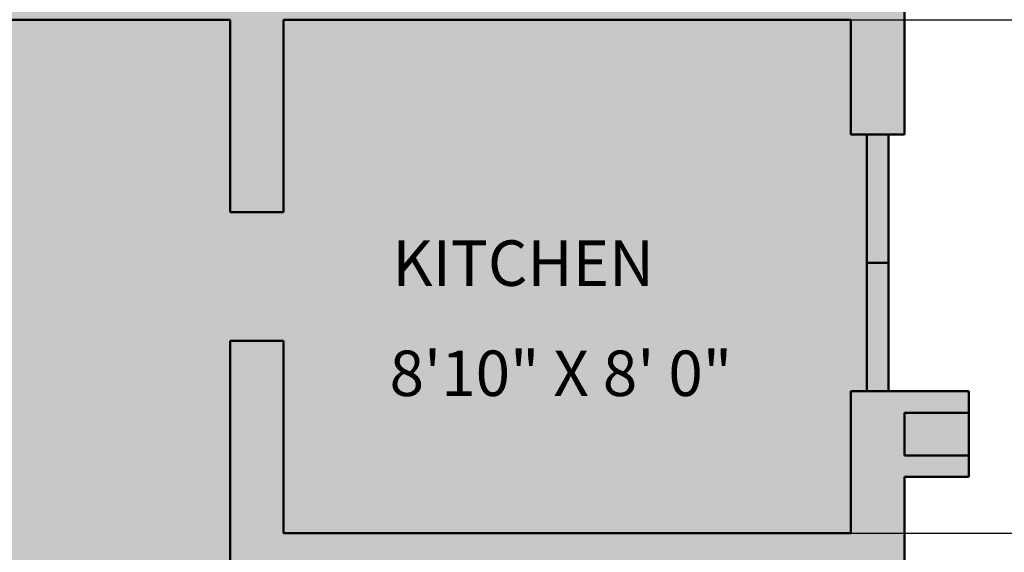
# Model space of a CAD drawing. Units: inches. Extents: x 925 to 2834, y 111 to 1355.
# Tile 19 of 25: x 1553 to 1737, y 972 to 1072. Entities that reach past the tile are written whole.
import ezdxf

# ---------------------------------------------------------------- set-up
doc = ezdxf.new("R2010")
doc.units = ezdxf.units.IN
doc.header["$MEASUREMENT"] = 0
for name, color, linetype, lineweight in [('A-ANNO-DIMS', 2, 'Continuous', 18), ('A-AREA-IDEN', 7, 'Continuous', 18), ('A-FLOR-PATT', 252, 'Continuous', 13), ('A-WALL', 7, 'Continuous', 50), ('A-WALL-PATT', 8, 'Continuous', 13)]:
    doc.layers.add(name, color=color, linetype=linetype, lineweight=lineweight)
doc.styles.get("Standard").update_dxf_attribs({"font": 'arial.ttf'})
doc.dimstyles.get("Standard").update_dxf_attribs({"dimtxt": 6, "dimasz": 3, "dimexe": 0.18, "dimexo": 0.0625, "dimgap": 0.09, "dimtad": 0, "dimtih": 1, "dimtoh": 1, "dimdec": 1, "dimzin": 0, "dimdsep": 46, "dimlunit": 3, "dimtxsty": 'Standard', "dimblk": 'ARCHTICK', "dimcen": 0.09, "dimadec": 0, "dimazin": 0, "dimtfac": 1, "dimtdec": 1, "dimtofl": 0, "dimtmove": 0, "dimatfit": 3, "dimfxl": 1, "dimtolj": 1, "dimtzin": 0, "dimarcsym": 0})

# ---------------------------------------------------------------- blocks, each defined once
blk = doc.blocks.new('_ArchTick')
at = {"color": 0, "linetype": 'ByBlock', "const_width": 0.15}
blk.add_lwpolyline([(-0.5, -0.5), (0.5, 0.5)], dxfattribs=at)
blk = doc.blocks.new('*D48')
at = {"layer": 'A-ANNO-DIMS', "color": 0, "lineweight": -2, "transparency": 16777216}
for p, q in [((1708.78, 975.59), (1988.62, 975.59)), ((1988.44, 975.59), (1988.44, 942.69)), ((1988.44, 903.59), (1988.44, 936.49)), ((1708.78, 903.59), (1988.62, 903.59))]:
    blk.add_line(p, q, dxfattribs=at)
at = {"layer": 'Defpoints', "color": 0, "transparency": 16777216}
for p in [(1708.71, 975.59), (1988.44, 975.59), (1708.71, 903.59)]:
    blk.add_point(p, dxfattribs=at)
at = {"layer": 'A-ANNO-DIMS', "color": 0, "lineweight": -2, "transparency": 16777216, "xscale": 3, "yscale": 3, "zscale": 3}
for p, rotation in [((1988.44, 975.59), 90), ((1988.44, 903.59), 270)]:
    blk.add_blockref('_ArchTick', p, dxfattribs=dict(at, rotation=rotation))
at = {"layer": 'A-ANNO-DIMS', "color": 0, "transparency": 16777216, "insert": (1988.44, 939.59), "char_height": 6, "attachment_point": 5}
blk.add_mtext('\\A1;72', dxfattribs=at)
blk = doc.blocks.new('*D49')
at = {"layer": 'A-ANNO-DIMS', "color": 0, "lineweight": -2, "transparency": 16777216}
for p, q in [((1708.78, 1071.59), (1988.62, 1071.59)), ((1988.44, 1071.59), (1988.44, 1026.74)), ((1988.44, 975.59), (1988.44, 1020.44)), ((1708.78, 975.59), (1988.62, 975.59))]:
    blk.add_line(p, q, dxfattribs=at)
at = {"layer": 'Defpoints', "color": 0, "transparency": 16777216}
for p in [(1708.71, 1071.59), (1988.44, 1071.59), (1708.71, 975.59)]:
    blk.add_point(p, dxfattribs=at)
at = {"layer": 'A-ANNO-DIMS', "color": 0, "lineweight": -2, "transparency": 16777216, "xscale": 3, "yscale": 3, "zscale": 3}
for p, rotation in [((1988.44, 1071.59), 90), ((1988.44, 975.59), 270)]:
    blk.add_blockref('_ArchTick', p, dxfattribs=dict(at, rotation=rotation))
at = {"layer": 'A-ANNO-DIMS', "color": 0, "transparency": 16777216, "insert": (1988.44, 1023.59), "char_height": 6, "attachment_point": 5}
blk.add_mtext('\\A1;96', dxfattribs=at)
blk = doc.blocks.new('*D50')
at = {"layer": 'A-ANNO-DIMS', "color": 0, "lineweight": -2, "transparency": 16777216}
for p, q in [((1718.78, 1081.59), (1988.62, 1081.59)), ((1988.44, 1081.59), (1988.44, 1079.74)), ((1988.44, 1071.59), (1988.44, 1073.44)), ((1708.78, 1071.59), (1988.62, 1071.59))]:
    blk.add_line(p, q, dxfattribs=at)
at = {"layer": 'Defpoints', "color": 0, "transparency": 16777216}
for p in [(1718.71, 1081.59), (1988.44, 1081.59), (1708.71, 1071.59)]:
    blk.add_point(p, dxfattribs=at)
at = {"layer": 'A-ANNO-DIMS', "color": 0, "lineweight": -2, "transparency": 16777216, "xscale": 3, "yscale": 3, "zscale": 3}
for p, rotation in [((1988.44, 1081.59), 90), ((1988.44, 1071.59), 270)]:
    blk.add_blockref('_ArchTick', p, dxfattribs=dict(at, rotation=rotation))
at = {"layer": 'A-ANNO-DIMS', "color": 0, "transparency": 16777216, "insert": (1988.44, 1076.59), "char_height": 6, "attachment_point": 5}
blk.add_mtext('\\A1;10', dxfattribs=at)

msp = doc.modelspace()

# ---------------------------------------------------------------- hatches: boundary and pattern name
at = {"layer": 'A-FLOR-PATT', "transparency": 33554605}
h = msp.add_hatch(color=256, dxfattribs=at)
h.dxf.hatch_style = 1
h.paths.add_polyline_path([(1931.688, 1294.5638), (991.7375, 1294.5638), (991.7375, 172.1134), (1931.688, 172.1134)])
h.paths.add_polyline_path([(1910.7128, 1273.5886), (1910.7128, 193.0886), (1012.7128, 193.0886), (1012.7128, 1273.5886)], flags=16)
h.paths.add_polyline_path([(1850.7128, 1213.5886), (1850.7128, 253.0886), (1072.7128, 253.0886), (1072.7128, 1213.5886)], flags=0)
h.paths.add_polyline_path([(1838.7128, 1201.5886), (1838.7128, 265.0886), (1084.7128, 265.0886), (1084.7128, 530.5886), (1084.7128, 1201.5886)], flags=0)
h.paths.add_polyline_path([(1547.6758, 1155.7396), (1547.6758, 1119.115), (1513.0687, 1119.115), (1513.0687, 1155.7396)], flags=0)
h.paths.add_polyline_path([(1600.1067, 1154.9439), (1634.7139, 1154.9439), (1634.7139, 1119.115), (1600.1067, 1119.115)], flags=0)
h.paths.add_polyline_path([(1505.2502, 1144.5358), (1505.2502, 1119.115), (1470.643, 1119.115), (1470.643, 1144.5358)], flags=0)
h.paths.add_polyline_path([(1559.1357, 1141.0962), (1593.7428, 1141.0962), (1593.7428, 1119.115), (1559.1357, 1119.115)], flags=0)
h.paths.add_polyline_path([(1462.8966, 1154.9439), (1462.8966, 1119.115), (1428.2895, 1119.115), (1428.2895, 1154.9439)], flags=0)
h.paths.add_polyline_path([(1642.4603, 1144.5358), (1677.0675, 1144.5358), (1677.0675, 1119.115), (1642.4603, 1119.115)], flags=0)
h.paths.add_polyline_path([(1422.3508, 1141.0962), (1422.3508, 1119.115), (1387.7436, 1119.115), (1387.7436, 1141.0962)], flags=0)
h.paths.add_polyline_path([(1684.8859, 1155.7396), (1719.4931, 1155.7396), (1719.4931, 1119.115), (1684.8859, 1119.115)], flags=0)
h.paths.add_polyline_path([(1718.7128, 1081.5886), (1718.7128, 1050.1249), (1715.7128, 1050.1249), (1715.7128, 1026.1249), (1715.7128, 1002.1249), (1718.7128, 1002.1249), (1730.7128, 1002.1249), (1730.7128, 998.1249), (1730.7128, 990.1249), (1730.7128, 986.1249), (1718.7128, 986.1249), (1718.7128, 893.5886), (1715.3735, 893.5886), (1715.3735, 891.5886), (1713.3735, 891.5886, 0.41421356), (1677.3735, 855.5886), (1713.3735, 855.5886), (1713.3735, 853.5886), (1715.3735, 853.5886), (1715.3735, 851.5886), (1718.7128, 851.5886), (1718.7128, 821.5865), (1734.4655, 821.5865), (1734.3735, 819.5886, -0.41421356), (1712.4415, 793.5886), (1712.4415, 791.5886), (1718.7128, 791.5886), (1718.7128, 717.5886), (1718.7128, 669.5886), (1732.7128, 669.5886), (1732.7128, 665.5886), (1732.7128, 641.5886), (1732.7128, 634.5886), (1732.7128, 610.5886), (1732.7128, 603.5886), (1718.7128, 603.5886), (1718.7128, 385.0886), (1434.2128, 385.0886), (1434.2128, 530.5886), (1410.2128, 530.5886), (1408.2128, 530.5886), (1408.2128, 532.5886, 0.41421356), (1372.2128, 568.5886), (1372.2128, 532.5886), (1370.2128, 532.5886), (1370.2128, 530.5886), (1368.2128, 530.5886), (1282.2128, 530.5886), (1210.2128, 530.5886), (1200.2128, 530.5886), (1200.2128, 542.1915), (1183.2307, 542.1915), (1183.2307, 546.1915), (1200.2128, 546.1915), (1200.2128, 572.1915), (1183.2307, 572.1915), (1183.2307, 576.1915), (1200.2128, 576.1915), (1200.2128, 727.5886), (1210.2128, 727.5886), (1234.2128, 727.5886), (1259.7128, 727.5886), (1259.7128, 775.5886), (1259.7128, 799.5886), (1259.7128, 847.5886), (1259.7128, 993.5872), (1259.7128, 1065.5872), (1259.7128, 1071.5886), (1219.6318, 1071.5886), (1219.6318, 1081.5886), (1084.7128, 1081.5886), (1084.7128, 1119.115), (1256.8974, 1119.115), (1256.8974, 1154.9439), (1291.5046, 1154.9439), (1291.5046, 1119.115), (1256.8974, 1119.115), (1256.6723, 1081.5886), (1293.7128, 1081.5886), (1341.7128, 1081.5886), (1341.7128, 1093.5886), (1347.7128, 1093.5886), (1371.7128, 1093.5886), (1377.7128, 1093.5886), (1377.7128, 1081.5886), (1668.7128, 1081.5886), (1668.7128, 1117.5886), (1675.7128, 1117.5886), (1711.7128, 1117.5886), (1718.7128, 1117.5886)], flags=0)
h.paths.add_polyline_path([(1376.2838, 1155.7396), (1376.2838, 1119.115), (1341.6766, 1119.115), (1341.6766, 1155.7396)], flags=0)
h.paths.add_polyline_path([(1341.7128, 1076.0886), (1293.7128, 1076.0886), (1293.7128, 1071.5886), (1269.7128, 1071.5886), (1269.7128, 1065.5872), (1266.7128, 1065.5872), (1266.7128, 1029.5872), (1265.7128, 1029.5872), (1265.7128, 993.5872), (1269.7128, 993.5872), (1269.7128, 903.5886), (1269.7128, 893.5886), (1269.7128, 847.5886), (1265.2128, 847.5886), (1265.2128, 799.5886), (1269.7128, 799.5886), (1269.7128, 775.5886), (1265.2128, 775.5886), (1265.2128, 727.5886), (1269.7128, 727.5886), (1444.2128, 727.5886), (1444.2128, 717.5886), (1234.2128, 717.5886), (1234.2128, 722.0886), (1210.2128, 722.0886), (1210.2128, 717.5886), (1210.2128, 540.5886), (1210.2128, 536.0886), (1282.2128, 536.0886), (1282.2128, 535.0886), (1210.2128, 535.0886), (1210.2128, 540.5886), (1210.2128, 717.5886), (1210.2128, 723.0886), (1234.2128, 723.0886), (1234.2128, 717.5886), (1444.2128, 717.5886), (1444.2128, 727.5886), (1269.7128, 727.5886), (1264.2128, 727.5886), (1264.2128, 775.5886), (1269.7128, 775.5886), (1269.7128, 799.5886), (1264.2128, 799.5886), (1264.2128, 847.5886), (1269.7128, 847.5886), (1269.7128, 893.5886), (1269.7128, 903.5886), (1269.7128, 993.5872), (1264.7128, 993.5872), (1264.7128, 1029.5872), (1265.7128, 1029.5872), (1265.7128, 1065.5872), (1269.7128, 1065.5872), (1269.7128, 1071.5886), (1293.7128, 1071.5886), (1293.7128, 1077.0886), (1341.7128, 1077.0886)], flags=0)
h.paths.add_polyline_path([(1730.9529, 1141.0962), (1765.5601, 1141.0962), (1765.5601, 1119.115), (1730.9529, 1119.115)], flags=0)
h.paths.add_polyline_path([(1333.8582, 1144.5358), (1333.8582, 1119.115), (1299.251, 1119.115), (1299.251, 1144.5358)], flags=0)
h.paths.add_polyline_path([(1592.7128, 968.5886), (1596.0342, 968.5886), (1602.7128, 968.5886), (1708.7128, 968.5886), (1708.7128, 903.5886), (1602.7128, 903.5886), (1602.7128, 938.5886), (1592.7128, 938.5886), (1592.7128, 903.5886), (1451.7128, 903.5886), (1451.7128, 893.5886), (1511.7128, 893.5886), (1511.7128, 881.5886), (1515.2128, 881.5886), (1518.7128, 881.5886), (1518.7128, 893.5886), (1592.7128, 893.5886), (1592.7128, 799.5886), (1518.7128, 799.5886), (1518.7128, 857.5886), (1511.7128, 857.5886), (1511.7128, 799.5886), (1511.7128, 772.0886), (1521.7128, 772.0886), (1521.7128, 792.5886), (1592.7128, 792.5886), (1592.7128, 727.5886), (1521.7128, 727.5886), (1521.7128, 748.0886), (1511.7128, 748.0886), (1511.7128, 717.5886), (1708.7128, 717.5886), (1714.2128, 717.5886), (1714.2128, 669.5886), (1708.7128, 669.5886), (1708.7128, 641.5886), (1492.2128, 641.5886), (1492.2128, 631.5886), (1621.2128, 631.5886), (1621.2128, 443.0886), (1625.7128, 443.0886), (1625.7128, 503.0886), (1625.7128, 507.5886), (1625.7128, 631.5886), (1708.7128, 631.5886), (1708.7128, 507.5886), (1655.7128, 507.5886), (1655.7128, 503.0886), (1708.7128, 503.0886), (1708.7128, 395.0886), (1625.7128, 395.0886), (1625.7128, 419.0886), (1621.2128, 419.0886), (1621.2128, 395.0886), (1482.2128, 395.0886), (1482.2128, 385.0886), (1434.2128, 385.0886), (1434.2128, 433.0886), (1444.2128, 433.0886), (1444.2128, 631.5886), (1450.2128, 631.5886), (1450.2128, 634.91), (1452.2128, 634.91), (1452.2128, 669.5886), (1454.2128, 669.5886, -0.40021217), (1490.1712, 635.3173), (1492.2128, 635.3173), (1492.2128, 641.5886), (1564.7128, 641.5886), (1564.7128, 677.5886), (1672.7128, 677.5886), (1672.7128, 681.5886), (1564.7128, 681.5886), (1564.7128, 717.5886), (1511.7128, 717.5886), (1511.7128, 748.0886), (1511.7128, 772.0886), (1511.7128, 799.5886), (1511.7128, 857.5886), (1511.8913, 857.5886), (1511.8913, 859.5886), (1515.6201, 859.5886, 0.41421356), (1537.552, 879.5886), (1513.552, 879.5886), (1511.8913, 879.5886), (1511.8913, 881.5886), (1511.7128, 881.5886), (1511.7128, 893.5886), (1451.7128, 893.5886), (1451.7128, 903.5886), (1592.7128, 903.5886), (1592.7128, 938.5886), (1592.7128, 940.5886), (1596.4415, 940.5886, 0.41421356), (1618.3735, 966.5886), (1594.3735, 966.5886), (1592.7128, 966.5886)], flags=0)
h.paths.add_polyline_path([(1377.7128, 903.5886), (1377.7128, 893.5886), (1305.7128, 893.5886), (1305.7128, 903.5886)], flags=0)
h.paths.add_polyline_path([(1708.7128, 821.5886), (1712.0342, 821.5886), (1712.0342, 819.5886), (1710.3735, 819.5886), (1708.7128, 819.5886)], flags=0)
h.paths.add_polyline_path([(1576.7128, 695.1992), (1575.5896, 693.6649), (1575.9687, 694.6994), (1575.4438, 695.1992), (1575.9687, 695.699), (1575.5896, 696.7335)], flags=0)
h.paths.add_polyline_path([(1565.9817, 662.3134), (1565.4568, 661.8136), (1565.8359, 660.7791), (1564.7128, 662.3134), (1565.8359, 663.8477), (1565.4568, 662.8132)], flags=0)
h.paths.add_polyline_path([(1444.2128, 433.0886), (1444.2128, 395.0886), (1482.2128, 395.0886), (1482.2128, 389.0886), (1438.2128, 389.0886), (1438.2128, 391.8608), (1438.2128, 433.0886)], flags=0)
h.paths.add_polyline_path([(1410.2128, 506.5886), (1410.2128, 289.0886), (1108.7128, 289.0886), (1108.7128, 506.5886)], flags=0)
h.paths.add_polyline_path([(1612.3153, 838.3016), (1680.4151, 838.3016), (1680.4151, 851.3131), (1612.3153, 851.3131)], flags=8)
h.paths.add_polyline_path([(1208.3174, 395.0436), (1282.1017, 395.0436), (1282.1017, 408.0552), (1208.3174, 408.0552)], flags=8)
h.paths.add_polyline_path([(1291.8049, 598.7427), (1369.8017, 598.7427), (1369.8017, 611.7542), (1291.8049, 611.7542)], flags=8)
h.paths.add_polyline_path([(1119.679, 917.3022), (1191.0817, 917.3022), (1191.0817, 930.3137), (1119.679, 930.3137)], flags=8)
h.paths.add_polyline_path([(1332.2261, 815.9808), (1410.2258, 815.9808), (1410.2258, 829.001), (1332.2261, 829.001)], flags=8)
h.paths.add_polyline_path([(1390.9013, 955.8158), (1475.4981, 955.8158), (1475.4981, 968.8273), (1390.9013, 968.8273)], flags=8)
h.paths.add_polyline_path([(1620.3436, 998.9325), (1688.4434, 998.9325), (1688.4434, 1011.944), (1620.3436, 1011.944)], flags=8)
h.paths.add_polyline_path([(1620.3436, 914.1039), (1691.7405, 914.1039), (1691.7405, 927.1155), (1620.3436, 927.1155)], flags=8)
h.paths.add_polyline_path([(1521.4542, 816.005), (1589.5569, 816.005), (1589.5569, 829.0253), (1521.4542, 829.0253)], flags=8)
h.paths.add_polyline_path([(1528.524, 740.3497), (1602.3082, 740.3497), (1602.3082, 753.3613), (1528.524, 753.3613)], flags=8)
h.paths.add_polyline_path([(1627.6094, 762.6128), (1702.3091, 762.6128), (1702.3091, 775.6244), (1627.6094, 775.6244)], flags=8)
h.paths.add_polyline_path([(1610.5442, 657.2751), (1684.3284, 657.2751), (1684.3284, 670.2867), (1610.5442, 670.2867)], flags=8)
h.paths.add_polyline_path([(1636.6983, 519.472), (1711.3981, 519.472), (1711.3981, 532.4835), (1636.6983, 532.4835)], flags=8)
h.paths.add_polyline_path([(1616.8577, 424.8539), (1694.8545, 424.8539), (1694.8545, 437.8654), (1616.8577, 437.8654)], flags=8)
h.paths.add_polyline_path([(1506.1456, 460.8838), (1579.9299, 460.8838), (1579.9299, 473.8953), (1506.1456, 473.8953)], flags=8)
h.paths.add_polyline_path([(1624.6119, 784.6011), (1696.9185, 784.6011), (1696.9185, 797.7864), (1624.6119, 797.7864)], flags=8)
h.paths.add_polyline_path([(1606.3732, 854.2194), (1683.3039, 854.2194), (1683.3039, 867.4048), (1606.3732, 867.4048)], flags=8)
h.paths.add_polyline_path([(1127.8008, 940.3581), (1165.1637, 940.3581), (1165.1637, 953.5348), (1127.8008, 953.5348)], flags=8)
h.paths.add_polyline_path([(1620.8657, 1019.4968), (1677.3447, 1019.4968), (1677.3447, 1032.6735), (1620.8657, 1032.6735)], flags=8)
h.paths.add_polyline_path([(1620.8643, 930.1821), (1703.0564, 930.1821), (1703.0564, 943.3675), (1620.8643, 943.3675)], flags=8)
h.paths.add_polyline_path([(1324.5702, 836.8338), (1408.0892, 836.8338), (1408.0892, 850.0191), (1324.5702, 850.0191)], flags=8)
h.paths.add_polyline_path([(1281.6584, 622.8885), (1383.6213, 622.8885), (1383.6213, 636.0739), (1281.6584, 636.0739)], flags=8)
h.paths.add_polyline_path([(1210.6721, 416.7893), (1269.1299, 416.7893), (1269.1299, 429.9747), (1210.6721, 429.9747)], flags=8)
h.paths.add_polyline_path([(1507.8264, 477.4836), (1586.7329, 477.4836), (1586.7329, 490.669), (1507.8264, 490.669)], flags=8)
h.paths.add_polyline_path([(1643.6238, 443.8135), (1696.6696, 443.8135), (1696.6696, 456.5643), (1643.6238, 456.5643)], flags=8)
h.paths.add_polyline_path([(1647.2466, 540.5638), (1693.1825, 540.5638), (1693.1825, 553.7491), (1647.2466, 553.7491)], flags=8)
h.paths.add_polyline_path([(1626.0633, 668.5064), (1673.3174, 668.5064), (1673.3174, 681.6831), (1626.0633, 681.6831)], flags=8)
h.paths.add_polyline_path([(1538.2915, 830.7872), (1567.5942, 830.7872), (1567.5942, 843.5293), (1538.2915, 843.5293)], flags=8)
h.paths.add_polyline_path([(1530.9338, 754.0477), (1559.576, 754.0477), (1559.576, 766.7898), (1530.9338, 766.7898)], flags=8)
h.paths.add_polyline_path([(1351.2461, 979.2309), (1513.8919, 979.2309), (1513.8919, 992.4076), (1351.2461, 992.4076)], flags=8)
at = {"layer": 'A-FLOR-PATT'}
h = msp.add_hatch(color=256, dxfattribs=at)
h.dxf.hatch_style = 1
h.paths.add_polyline_path([(1850.7128, 1213.5886), (1072.7128, 1213.5886), (1072.7128, 253.0886), (1850.7128, 253.0886)])
h.paths.add_polyline_path([(1084.7128, 1201.5886), (1838.7128, 1201.5886), (1838.7128, 265.0886), (1084.7128, 265.0886)], flags=16)
h.paths.add_polyline_path([(1183.2307, 576.1915), (1200.2128, 576.1915), (1200.2128, 727.5886), (1210.2128, 727.5886), (1234.2128, 727.5886), (1259.7128, 727.5886), (1259.7128, 775.5886), (1259.7128, 799.5886), (1259.7128, 847.5886), (1259.7128, 993.5872), (1259.7128, 1065.5872), (1259.7128, 1071.5886), (1219.6318, 1071.5886), (1219.6318, 1081.5886), (1293.7128, 1081.5886), (1341.7128, 1081.5886), (1341.7128, 1093.5886), (1347.7128, 1093.5886), (1347.7128, 1081.5886), (1371.7128, 1081.5886), (1371.7128, 1093.5886), (1377.7128, 1093.5886), (1377.7128, 1081.5886), (1668.7128, 1081.5886), (1668.7128, 1117.5886), (1675.7128, 1117.5886), (1675.7128, 1081.5886), (1711.7128, 1081.5886), (1711.7128, 1117.5886), (1718.7128, 1117.5886), (1718.7128, 1081.5886), (1718.7128, 1050.1249), (1715.7128, 1050.1249), (1715.7128, 1026.1249), (1715.7128, 1002.1249), (1718.7128, 1002.1249), (1730.7128, 1002.1249), (1730.7128, 998.1249), (1730.7128, 990.1249), (1730.7128, 986.1249), (1718.7128, 986.1249), (1718.7128, 893.5886), (1715.3735, 893.5886), (1715.3735, 891.5886), (1713.3735, 891.5886, 0.41421356), (1677.3735, 855.5886), (1713.3735, 855.5886), (1713.3735, 853.5886), (1715.3735, 853.5886), (1715.3735, 851.5886), (1718.7128, 851.5886), (1718.7128, 821.5865), (1734.4655, 821.5865), (1734.3735, 819.5886, -0.41421356), (1712.4415, 793.5886), (1712.4415, 791.5886), (1718.7128, 791.5886), (1718.7128, 717.5886), (1718.7128, 669.5886), (1732.7128, 669.5886), (1732.7128, 665.5886), (1732.7128, 641.5886), (1732.7128, 634.5886), (1732.7128, 610.5886), (1732.7128, 603.5886), (1718.7128, 603.5886), (1718.7128, 385.0886), (1434.2128, 385.0886), (1434.2128, 433.0886), (1434.2128, 530.5886), (1410.2128, 530.5886), (1408.2128, 530.5886), (1408.2128, 532.5886, 0.41421356), (1372.2128, 568.5886), (1372.2128, 532.5886), (1370.2128, 532.5886), (1370.2128, 530.5886), (1368.2128, 530.5886), (1282.2128, 530.5886), (1210.2128, 530.5886), (1200.2128, 530.5886), (1200.2128, 542.1915), (1183.2307, 542.1915), (1183.2307, 546.1915), (1200.2128, 546.1915), (1200.2128, 572.1915), (1183.2307, 572.1915)], flags=0)
h.paths.add_polyline_path([(1210.2128, 717.5886), (1210.2128, 723.0886), (1234.2128, 723.0886), (1234.2128, 717.5886), (1444.2128, 717.5886), (1444.2128, 727.5886), (1269.7128, 727.5886), (1264.2128, 727.5886), (1264.2128, 775.5886), (1269.7128, 775.5886), (1269.7128, 799.5886), (1264.2128, 799.5886), (1264.2128, 847.5886), (1269.7128, 847.5886), (1269.7128, 893.5886), (1269.7128, 903.5886), (1269.7128, 993.5872), (1264.7128, 993.5872), (1264.7128, 1029.5872), (1265.7128, 1029.5872), (1265.7128, 1065.5872), (1269.7128, 1065.5872), (1269.7128, 1071.5886), (1293.7128, 1071.5886), (1293.7128, 1077.0886), (1341.7128, 1077.0886), (1341.7128, 1076.0886), (1293.7128, 1076.0886), (1293.7128, 1071.5886), (1269.7128, 1071.5886), (1269.7128, 1065.5872), (1266.7128, 1065.5872), (1266.7128, 1029.5872), (1265.7128, 1029.5872), (1265.7128, 993.5872), (1269.7128, 993.5872), (1269.7128, 903.5886), (1269.7128, 893.5886), (1269.7128, 847.5886), (1265.2128, 847.5886), (1265.2128, 799.5886), (1269.7128, 799.5886), (1269.7128, 775.5886), (1265.2128, 775.5886), (1265.2128, 727.5886), (1269.7128, 727.5886), (1444.2128, 727.5886), (1444.2128, 717.5886), (1234.2128, 717.5886), (1234.2128, 722.0886), (1210.2128, 722.0886), (1210.2128, 717.5886), (1210.2128, 540.5886), (1210.2128, 536.0886), (1282.2128, 536.0886), (1282.2128, 535.0886), (1210.2128, 535.0886), (1210.2128, 540.5886)], flags=0)
h.paths.add_polyline_path([(1450.2128, 634.91), (1452.2128, 634.91), (1452.2128, 669.5886), (1454.2128, 669.5886, -0.40021217), (1490.1712, 635.3173), (1492.2128, 635.3173), (1492.2128, 641.5886), (1564.7128, 641.5886), (1564.7128, 677.5886), (1672.7128, 677.5886), (1672.7128, 681.5886), (1564.7128, 681.5886), (1564.7128, 717.5886), (1511.7128, 717.5886), (1511.7128, 748.0886), (1511.7128, 772.0886), (1511.7128, 799.5886), (1511.7128, 857.5886), (1511.8913, 857.5886), (1511.8913, 859.5886), (1515.6201, 859.5886, 0.41421356), (1537.552, 879.5886), (1513.552, 879.5886), (1511.8913, 879.5886), (1511.8913, 881.5886), (1511.7128, 881.5886), (1511.7128, 893.5886), (1451.7128, 893.5886), (1451.7128, 903.5886), (1592.7128, 903.5886), (1592.7128, 938.5886), (1592.7128, 940.5886), (1596.4415, 940.5886, 0.41421356), (1618.3735, 966.5886), (1594.3735, 966.5886), (1592.7128, 966.5886), (1592.7128, 968.5886), (1596.0342, 968.5886), (1602.7128, 968.5886), (1708.7128, 968.5886), (1708.7128, 903.5886), (1602.7128, 903.5886), (1602.7128, 938.5886), (1592.7128, 938.5886), (1592.7128, 903.5886), (1451.7128, 903.5886), (1451.7128, 893.5886), (1511.7128, 893.5886), (1511.7128, 881.5886), (1518.7128, 881.5886), (1518.7128, 893.5886), (1592.7128, 893.5886), (1592.7128, 799.5886), (1518.7128, 799.5886), (1518.7128, 857.5886), (1511.7128, 857.5886), (1511.7128, 799.5886), (1511.7128, 772.0886), (1521.7128, 772.0886), (1521.7128, 792.5886), (1592.7128, 792.5886), (1592.7128, 727.5886), (1521.7128, 727.5886), (1521.7128, 748.0886), (1511.7128, 748.0886), (1511.7128, 717.5886), (1708.7128, 717.5886), (1714.2128, 717.5886), (1714.2128, 669.5886), (1708.7128, 669.5886), (1708.7128, 641.5886), (1492.2128, 641.5886), (1492.2128, 631.5886), (1621.2128, 631.5886), (1621.2128, 443.0886), (1625.7128, 443.0886), (1625.7128, 503.0886), (1625.7128, 507.5886), (1625.7128, 631.5886), (1708.7128, 631.5886), (1708.7128, 507.5886), (1655.7128, 507.5886), (1655.7128, 503.0886), (1708.7128, 503.0886), (1708.7128, 395.0886), (1625.7128, 395.0886), (1625.7128, 419.0886), (1621.2128, 419.0886), (1621.2128, 395.0886), (1482.2128, 395.0886), (1482.2128, 389.0886), (1438.2128, 389.0886), (1438.2128, 391.8608), (1438.2128, 433.0886), (1444.2128, 433.0886), (1444.2128, 631.5886), (1450.2128, 631.5886)], flags=0)
h.paths.add_polyline_path([(1444.2128, 433.0886), (1444.2128, 395.0886), (1482.2128, 395.0886), (1482.2128, 391.0886), (1440.2128, 391.0886), (1440.2128, 391.8608), (1440.2128, 433.0886)], flags=0)
h.paths.add_polyline_path([(1305.7128, 893.5886), (1305.7128, 903.5886), (1377.7128, 903.5886), (1377.7128, 893.5886)], flags=0)
h.paths.add_polyline_path([(1564.7128, 662.3134), (1565.8359, 663.8477), (1565.4568, 662.8132), (1565.9817, 662.3134), (1565.4568, 661.8136), (1565.8359, 660.7791)], flags=0)
h.paths.add_polyline_path([(1575.4438, 695.1992), (1575.9687, 695.699), (1575.5896, 696.7335), (1576.7128, 695.1992), (1575.5896, 693.6649), (1575.9687, 694.6994)], flags=0)
h.paths.add_polyline_path([(1708.7128, 821.5886), (1712.0342, 821.5886), (1712.0342, 819.5886), (1710.3735, 819.5886), (1708.7128, 819.5886)], flags=0)
h = msp.add_hatch(color=256, dxfattribs=at)
h.dxf.hatch_style = 1
h.paths.add_polyline_path([(1718.7128, 603.5886), (1708.7128, 603.5886), (1708.7128, 507.5886), (1655.7128, 507.5886), (1655.7128, 503.0886), (1708.7128, 503.0886), (1708.7128, 395.0886), (1625.7128, 395.0886), (1625.7128, 419.0886), (1621.2128, 419.0886), (1621.2128, 395.0886), (1482.2128, 395.0886), (1482.2128, 385.0886), (1718.7128, 385.0886)])
h.paths.add_polyline_path([(1625.7128, 631.5886), (1708.7128, 631.5886), (1708.7128, 603.5886), (1718.7128, 603.5886), (1732.7128, 603.5886), (1732.7128, 610.5886), (1715.7128, 610.5886), (1715.7128, 634.5886), (1732.7128, 634.5886), (1732.7128, 641.5886), (1715.7128, 641.5886), (1715.7128, 665.5886), (1732.7128, 665.5886), (1732.7128, 669.5886), (1708.7128, 669.5886), (1708.7128, 641.5886), (1492.2128, 641.5886), (1492.2128, 631.5886), (1621.2128, 631.5886), (1621.2128, 443.0886), (1625.7128, 443.0886), (1625.7128, 503.0886), (1625.7128, 507.5886)])
h.paths.add_polyline_path([(1718.7128, 851.5886), (1708.7128, 851.5886), (1708.7128, 828.5886), (1602.7128, 828.5886), (1602.7128, 893.5886), (1708.7128, 893.5886), (1718.7128, 893.5886), (1718.7128, 986.1249), (1730.7128, 986.1249), (1730.7128, 990.1249), (1718.7128, 990.1249), (1718.7128, 998.1249), (1730.7128, 998.1249), (1730.7128, 1002.1249), (1718.7128, 1002.1249), (1708.7128, 1002.1249), (1708.7128, 975.5886), (1602.7128, 975.5886), (1602.7128, 1011.5886), (1592.7128, 1011.5886), (1592.7128, 968.5886), (1596.0342, 968.5886), (1602.7128, 968.5886), (1708.7128, 968.5886), (1708.7128, 903.5886), (1602.7128, 903.5886), (1602.7128, 938.5886), (1592.7128, 938.5886), (1592.7128, 903.5886), (1451.7128, 903.5886), (1451.7128, 893.5886), (1511.7128, 893.5886), (1511.7128, 881.5886), (1515.2128, 881.5886), (1518.7128, 881.5886), (1518.7128, 893.5886), (1592.7128, 893.5886), (1592.7128, 799.5886), (1518.7128, 799.5886), (1518.7128, 857.5886), (1511.7128, 857.5886), (1511.7128, 799.5886), (1511.7128, 772.0886), (1521.7128, 772.0886), (1521.7128, 792.5886), (1592.7128, 792.5886), (1592.7128, 727.5886), (1521.7128, 727.5886), (1521.7128, 748.0886), (1511.7128, 748.0886), (1511.7128, 717.5886), (1708.7128, 717.5886), (1718.7128, 717.5886), (1718.7128, 727.5886), (1718.7128, 791.5886), (1708.7128, 791.5886), (1708.7128, 727.5886), (1602.7128, 727.5886), (1602.7128, 821.5886), (1708.7128, 821.5886), (1712.0342, 821.5886), (1718.7128, 821.5886)])
h.paths.add_polyline_path([(1718.7128, 1081.5886), (1718.7128, 1117.5886), (1711.7128, 1117.5886), (1711.7128, 1081.5886), (1675.7128, 1081.5886), (1675.7128, 1117.5886), (1668.7128, 1117.5886), (1668.7128, 1081.5886), (1377.7128, 1081.5886), (1377.7128, 1093.5886), (1371.7128, 1093.5886), (1371.7128, 1081.5886), (1347.7128, 1081.5886), (1347.7128, 1093.5886), (1341.7128, 1093.5886), (1341.7128, 1081.5886), (1341.7128, 1071.5886), (1592.7128, 1071.5886), (1592.7128, 1035.5886), (1602.7128, 1035.5886), (1602.7128, 1071.5886), (1708.7128, 1071.5886), (1708.7128, 1050.1249), (1718.7128, 1050.1249)])
h.paths.add_polyline_path([(1293.7128, 1081.5886), (1219.6318, 1081.5886), (1219.6318, 1071.5886), (1259.7128, 1071.5886), (1259.7128, 1065.5872), (1269.7128, 1065.5872), (1269.7128, 1071.5886), (1293.7128, 1071.5886)])
h.paths.add_polyline_path([(1269.7128, 903.5886), (1269.7128, 993.5872), (1259.7128, 993.5872), (1259.7128, 847.5886), (1269.7128, 847.5886), (1269.7128, 893.5886)])
h.paths.add_polyline_path([(1377.7128, 903.5886), (1305.7128, 903.5886), (1305.7128, 893.5886), (1377.7128, 893.5886)])
h.paths.add_polyline_path([(1444.2128, 727.5886), (1269.7128, 727.5886), (1259.7128, 727.5886), (1234.2128, 727.5886), (1234.2128, 717.5886), (1444.2128, 717.5886)])
h.paths.add_polyline_path([(1269.7128, 799.5886), (1259.7128, 799.5886), (1259.7128, 775.5886), (1269.7128, 775.5886)])
h.paths.add_polyline_path([(1444.2128, 631.5886), (1450.2128, 631.5886), (1450.2128, 634.91), (1450.2128, 641.5886), (1434.2128, 641.5886), (1434.2128, 540.5886), (1410.2128, 540.5886), (1410.2128, 530.5886), (1434.2128, 530.5886), (1434.2128, 433.0886), (1444.2128, 433.0886)])
h.paths.add_polyline_path([(1368.2128, 533.91), (1368.2128, 540.5886), (1282.2128, 540.5886), (1282.2128, 530.5886), (1368.2128, 530.5886)])
h.paths.add_polyline_path([(1210.2128, 717.5886), (1210.2128, 727.5886), (1200.2128, 727.5886), (1200.2128, 576.1915), (1183.2307, 576.1915), (1183.2307, 572.1915), (1200.2128, 572.1915), (1200.2128, 546.1915), (1183.2307, 546.1915), (1183.2307, 542.1915), (1200.2128, 542.1915), (1200.2128, 530.5886), (1210.2128, 530.5886), (1210.2128, 540.5886)])
at = {"layer": 'A-FLOR-PATT', "transparency": 33554605}
h = msp.add_hatch(color=256, dxfattribs=at)
h.dxf.hatch_style = 1
h.paths.add_polyline_path([(1592.7128, 938.5886), (1592.7128, 940.5886), (1596.4415, 940.5886, 0.41421356), (1618.3735, 966.5886), (1594.3735, 966.5886), (1592.7128, 966.5886), (1592.7128, 968.5886), (1592.7128, 1011.5886), (1602.7128, 1011.5886), (1602.7128, 975.5886), (1708.7128, 975.5886), (1708.7128, 1002.1249), (1711.7128, 1002.1249), (1711.7128, 1026.1249), (1711.7128, 1050.1249), (1708.7128, 1050.1249), (1708.7128, 1071.5886), (1602.7128, 1071.5886), (1602.7128, 1035.5886), (1592.7128, 1035.5886), (1592.7128, 1071.5886), (1341.7128, 1071.5886), (1293.7128, 1071.5886), (1269.7128, 1071.5886), (1269.7128, 1065.5872), (1269.7128, 993.5872), (1269.7128, 903.5886), (1269.7128, 893.5886), (1269.7128, 847.5886), (1269.7128, 799.5886), (1269.7128, 775.5886), (1269.7128, 727.5886), (1444.2128, 727.5886), (1444.2128, 717.5886), (1234.2128, 717.5886), (1210.2128, 717.5886), (1210.2128, 540.5886), (1282.2128, 540.5886), (1368.2128, 540.5886), (1368.2128, 533.91), (1370.2128, 533.91), (1370.2128, 568.5886), (1372.2128, 568.5886, -0.40021217), (1408.1712, 534.3173), (1410.2128, 534.3173), (1410.2128, 540.5886), (1434.2128, 540.5886), (1434.2128, 641.5886), (1450.2128, 641.5886), (1450.2128, 634.91), (1452.2128, 634.91), (1452.2128, 669.5886), (1454.2128, 669.5886, -0.40021217), (1490.1712, 635.3173), (1492.2128, 635.3173), (1492.2128, 641.5886), (1564.7128, 641.5886), (1564.7128, 677.5886), (1672.7128, 677.5886), (1672.7128, 681.5886), (1564.7128, 681.5886), (1564.7128, 717.5886), (1511.7128, 717.5886), (1511.7128, 748.0886), (1511.7128, 772.0886), (1511.7128, 799.5886), (1511.7128, 857.5886), (1511.8913, 857.5886), (1511.8913, 859.5886), (1515.6201, 859.5886, 0.41421356), (1537.552, 879.5886), (1513.552, 879.5886), (1511.8913, 879.5886), (1511.8913, 881.5886), (1511.7128, 881.5886), (1511.7128, 893.5886), (1451.7128, 893.5886), (1451.7128, 903.5886), (1592.7128, 903.5886)])
h.paths.add_polyline_path([(1377.7128, 903.5886), (1377.7128, 893.5886), (1305.7128, 893.5886), (1305.7128, 903.5886)], flags=16)
h.paths.add_polyline_path([(1592.7128, 893.5886), (1518.7128, 893.5886), (1518.7128, 881.5865), (1537.6441, 881.5865), (1537.552, 879.5886, -0.41421356), (1515.6201, 859.5886), (1515.6201, 857.5886), (1518.7128, 857.5886), (1518.7128, 799.5886), (1592.7128, 799.5886)], flags=17)
h.paths.add_polyline_path([(1291.8049, 598.7427), (1369.8017, 598.7427), (1369.8017, 611.7542), (1291.8049, 611.7542)], flags=24)
h.paths.add_polyline_path([(1332.2261, 815.9808), (1410.2258, 815.9808), (1410.2258, 829.001), (1332.2261, 829.001)], flags=24)
h.paths.add_polyline_path([(1390.9013, 955.8158), (1475.4981, 955.8158), (1475.4981, 968.8273), (1390.9013, 968.8273)], flags=24)
h.paths.add_polyline_path([(1620.3436, 998.9325), (1688.4434, 998.9325), (1688.4434, 1011.944), (1620.3436, 1011.944)], flags=24)
h.paths.add_polyline_path([(1620.8657, 1019.4968), (1677.3447, 1019.4968), (1677.3447, 1032.6735), (1620.8657, 1032.6735)], flags=24)
h.paths.add_polyline_path([(1324.5702, 836.8338), (1408.0892, 836.8338), (1408.0892, 850.0191), (1324.5702, 850.0191)], flags=24)
h.paths.add_polyline_path([(1281.6584, 622.8885), (1383.6213, 622.8885), (1383.6213, 636.0739), (1281.6584, 636.0739)], flags=24)
h.paths.add_polyline_path([(1626.0633, 668.5064), (1673.3174, 668.5064), (1673.3174, 681.6831), (1626.0633, 681.6831)], flags=25)
h.paths.add_polyline_path([(1351.2461, 979.2309), (1513.8919, 979.2309), (1513.8919, 992.4076), (1351.2461, 992.4076)], flags=24)
h.paths.add_polyline_path([(1521.4542, 816.005), (1589.5569, 816.005), (1589.5569, 829.0253), (1521.4542, 829.0253)], flags=24)
h.paths.add_polyline_path([(1538.2915, 830.7872), (1567.5942, 830.7872), (1567.5942, 843.5293), (1538.2915, 843.5293)], flags=24)
h.paths.add_polyline_path([(1636.6983, 519.472), (1711.3981, 519.472), (1711.3981, 532.4835), (1636.6983, 532.4835)], flags=9)
h.paths.add_polyline_path([(1616.8577, 424.8539), (1694.8545, 424.8539), (1694.8545, 437.8654), (1616.8577, 437.8654)], flags=9)
h.paths.add_polyline_path([(1506.1456, 460.8838), (1579.9299, 460.8838), (1579.9299, 473.8953), (1506.1456, 473.8953)], flags=9)
h.paths.add_polyline_path([(1606.3732, 854.2194), (1683.3039, 854.2194), (1683.3039, 867.4048), (1606.3732, 867.4048)], flags=25)
h.paths.add_polyline_path([(1507.8264, 477.4836), (1586.7329, 477.4836), (1586.7329, 490.669), (1507.8264, 490.669)], flags=9)
h.paths.add_polyline_path([(1643.6238, 443.8135), (1696.6696, 443.8135), (1696.6696, 456.5643), (1643.6238, 456.5643)], flags=9)
h.paths.add_polyline_path([(1647.2466, 540.5638), (1693.1825, 540.5638), (1693.1825, 553.7491), (1647.2466, 553.7491)], flags=25)
h = msp.add_hatch(color=256, dxfattribs=at)
h.dxf.hatch_style = 1
h.paths.add_polyline_path([(1200.2128, 727.5886), (1084.7128, 727.5886), (1084.7128, 530.5886), (1200.2128, 530.5886), (1200.2128, 542.1915), (1183.2307, 542.1915), (1183.2307, 546.1915), (1200.2128, 546.1915), (1200.2128, 572.1915), (1183.2307, 572.1915), (1183.2307, 576.1915), (1200.2128, 576.1915)])
h.paths.add_polyline_path([(1612.3153, 838.3016), (1680.4151, 838.3016), (1680.4151, 851.3131), (1612.3153, 851.3131)], flags=9)
h.paths.add_polyline_path([(1291.8049, 598.7427), (1369.8017, 598.7427), (1369.8017, 611.7542), (1291.8049, 611.7542)], flags=9)
h.paths.add_polyline_path([(1119.679, 917.3022), (1191.0817, 917.3022), (1191.0817, 930.3137), (1119.679, 930.3137)], flags=9)
h.paths.add_polyline_path([(1332.2261, 815.9808), (1410.2258, 815.9808), (1410.2258, 829.001), (1332.2261, 829.001)], flags=9)
h.paths.add_polyline_path([(1390.9013, 955.8158), (1475.4981, 955.8158), (1475.4981, 968.8273), (1390.9013, 968.8273)], flags=9)
h.paths.add_polyline_path([(1620.3436, 998.9325), (1688.4434, 998.9325), (1688.4434, 1011.944), (1620.3436, 1011.944)], flags=9)
h.paths.add_polyline_path([(1620.3436, 914.1039), (1691.7405, 914.1039), (1691.7405, 927.1155), (1620.3436, 927.1155)], flags=9)
h.paths.add_polyline_path([(1521.4542, 816.005), (1589.5569, 816.005), (1589.5569, 829.0253), (1521.4542, 829.0253)], flags=9)
h.paths.add_polyline_path([(1522.4337, 740.3497), (1596.218, 740.3497), (1596.218, 753.3613), (1522.4337, 753.3613)], flags=9)
h.paths.add_polyline_path([(1606.3732, 854.2194), (1683.3039, 854.2194), (1683.3039, 867.4048), (1606.3732, 867.4048)], flags=9)
h.paths.add_polyline_path([(1127.8008, 940.3581), (1165.1637, 940.3581), (1165.1637, 953.5348), (1127.8008, 953.5348)], flags=9)
h.paths.add_polyline_path([(1620.8657, 1019.4968), (1677.3447, 1019.4968), (1677.3447, 1032.6735), (1620.8657, 1032.6735)], flags=9)
h.paths.add_polyline_path([(1620.8643, 930.1821), (1703.0564, 930.1821), (1703.0564, 943.3675), (1620.8643, 943.3675)], flags=9)
h.paths.add_polyline_path([(1324.5702, 836.8338), (1408.0892, 836.8338), (1408.0892, 850.0191), (1324.5702, 850.0191)], flags=9)
h.paths.add_polyline_path([(1281.6584, 622.8885), (1383.6213, 622.8885), (1383.6213, 636.0739), (1281.6584, 636.0739)], flags=9)
h.paths.add_polyline_path([(1626.0633, 668.5064), (1673.3174, 668.5064), (1673.3174, 681.6831), (1626.0633, 681.6831)], flags=9)
h.paths.add_polyline_path([(1538.2915, 830.7872), (1567.5942, 830.7872), (1567.5942, 843.5293), (1538.2915, 843.5293)], flags=9)
h.paths.add_polyline_path([(1351.2461, 979.2309), (1513.8919, 979.2309), (1513.8919, 992.4076), (1351.2461, 992.4076)], flags=9)
h = msp.add_hatch(color=256, dxfattribs=at)
h.dxf.hatch_style = 1
h.paths.add_polyline_path([(1621.2128, 631.5886), (1492.2128, 631.5886), (1490.2128, 631.5886), (1490.2128, 633.5886, 0.41421356), (1454.2128, 669.5886), (1454.2128, 633.5886), (1452.2128, 633.5886), (1452.2128, 631.5886), (1450.2128, 631.5886), (1444.2128, 631.5886), (1444.2128, 395.0886), (1482.2128, 395.0886), (1621.2128, 395.0886), (1621.2128, 419.0886), (1625.7128, 419.0886), (1625.7128, 395.0886), (1708.7128, 395.0886), (1708.7128, 503.0886), (1655.7128, 503.0886), (1655.7128, 507.5886), (1708.7128, 507.5886), (1708.7128, 631.5886), (1625.7128, 631.5886), (1625.7128, 507.5886), (1625.7128, 503.0886), (1625.7128, 443.0886), (1621.2128, 443.0886)])
h.paths.add_polyline_path([(1636.6983, 519.472), (1711.3981, 519.472), (1711.3981, 532.4835), (1636.6983, 532.4835)], flags=9)
h.paths.add_polyline_path([(1616.8577, 424.8539), (1694.8545, 424.8539), (1694.8545, 437.8654), (1616.8577, 437.8654)], flags=24)
h.paths.add_polyline_path([(1506.1456, 460.8838), (1579.9299, 460.8838), (1579.9299, 473.8953), (1506.1456, 473.8953)], flags=24)
h.paths.add_polyline_path([(1507.8264, 477.4836), (1586.7329, 477.4836), (1586.7329, 490.669), (1507.8264, 490.669)], flags=24)
h.paths.add_polyline_path([(1643.6238, 443.8135), (1696.6696, 443.8135), (1696.6696, 456.5643), (1643.6238, 456.5643)], flags=24)
h.paths.add_polyline_path([(1647.2466, 540.5638), (1693.1825, 540.5638), (1693.1825, 553.7491), (1647.2466, 553.7491)], flags=24)
h.paths.add_polyline_path([(1612.3153, 838.3016), (1680.4151, 838.3016), (1680.4151, 851.3131), (1612.3153, 851.3131)], flags=9)
h.paths.add_polyline_path([(1291.8049, 598.7427), (1369.8017, 598.7427), (1369.8017, 611.7542), (1291.8049, 611.7542)], flags=9)
h.paths.add_polyline_path([(1119.679, 917.3022), (1191.0817, 917.3022), (1191.0817, 930.3137), (1119.679, 930.3137)], flags=9)
h.paths.add_polyline_path([(1332.2261, 815.9808), (1410.2258, 815.9808), (1410.2258, 829.001), (1332.2261, 829.001)], flags=9)
h.paths.add_polyline_path([(1390.9013, 955.8158), (1475.4981, 955.8158), (1475.4981, 968.8273), (1390.9013, 968.8273)], flags=9)
h.paths.add_polyline_path([(1620.3436, 998.9325), (1688.4434, 998.9325), (1688.4434, 1011.944), (1620.3436, 1011.944)], flags=9)
h.paths.add_polyline_path([(1620.3436, 914.1039), (1691.7405, 914.1039), (1691.7405, 927.1155), (1620.3436, 927.1155)], flags=9)
h.paths.add_polyline_path([(1521.4542, 816.005), (1589.5569, 816.005), (1589.5569, 829.0253), (1521.4542, 829.0253)], flags=9)
h.paths.add_polyline_path([(1528.524, 740.3497), (1602.3082, 740.3497), (1602.3082, 753.3613), (1528.524, 753.3613)], flags=9)
h.paths.add_polyline_path([(1627.6094, 762.6128), (1702.3091, 762.6128), (1702.3091, 775.6244), (1627.6094, 775.6244)], flags=9)
h.paths.add_polyline_path([(1624.6119, 784.6011), (1696.9185, 784.6011), (1696.9185, 797.7864), (1624.6119, 797.7864)], flags=9)
h.paths.add_polyline_path([(1606.3732, 854.2194), (1683.3039, 854.2194), (1683.3039, 867.4048), (1606.3732, 867.4048)], flags=9)
h.paths.add_polyline_path([(1127.8008, 940.3581), (1165.1637, 940.3581), (1165.1637, 953.5348), (1127.8008, 953.5348)], flags=9)
h.paths.add_polyline_path([(1620.8657, 1019.4968), (1677.3447, 1019.4968), (1677.3447, 1032.6735), (1620.8657, 1032.6735)], flags=9)
h.paths.add_polyline_path([(1620.8643, 930.1821), (1703.0564, 930.1821), (1703.0564, 943.3675), (1620.8643, 943.3675)], flags=9)
h.paths.add_polyline_path([(1324.5702, 836.8338), (1408.0892, 836.8338), (1408.0892, 850.0191), (1324.5702, 850.0191)], flags=9)
h.paths.add_polyline_path([(1281.6584, 622.8885), (1383.6213, 622.8885), (1383.6213, 636.0739), (1281.6584, 636.0739)], flags=9)
h.paths.add_polyline_path([(1626.0633, 668.5064), (1673.3174, 668.5064), (1673.3174, 681.6831), (1626.0633, 681.6831)], flags=9)
h.paths.add_polyline_path([(1538.2915, 830.7872), (1567.5942, 830.7872), (1567.5942, 843.5293), (1538.2915, 843.5293)], flags=9)
h.paths.add_polyline_path([(1530.9338, 754.0477), (1559.576, 754.0477), (1559.576, 766.7898), (1530.9338, 766.7898)], flags=9)
h.paths.add_polyline_path([(1351.2461, 979.2309), (1513.8919, 979.2309), (1513.8919, 992.4076), (1351.2461, 992.4076)], flags=9)
at = {"layer": 'A-WALL-PATT'}
h = msp.add_hatch(color=256, dxfattribs=at)
h.dxf.hatch_style = 1
h.paths.add_polyline_path([(1715.7128, 1050.1249), (1711.7128, 1050.1249), (1711.7128, 1026.1249), (1715.7128, 1026.1249)])
h.paths.add_polyline_path([(1715.7128, 1026.1249), (1711.7128, 1026.1249), (1711.7128, 1002.1249), (1715.7128, 1002.1249)])
at = {"layer": 'A-WALL-PATT', "transparency": 33554605}
h = msp.add_hatch(color=256, dxfattribs=at)
h.dxf.hatch_style = 1
h.paths.add_polyline_path([(1732.7128, 634.5886), (1715.7128, 634.5886), (1715.7128, 610.5886), (1732.7128, 610.5886)])
h.paths.add_polyline_path([(1732.7128, 665.5886), (1715.7128, 665.5886), (1715.7128, 641.5886), (1732.7128, 641.5886)])
h.paths.add_polyline_path([(1730.7128, 998.1249), (1718.7128, 998.1249), (1718.7128, 990.1249), (1730.7128, 990.1249)])

# ---------------------------------------------------------------- linework, layer by layer
at = {"layer": 'A-WALL'}
for p, q in [((1718.7128, 1081.5886), (1718.7128, 1050.1249)), ((1718.7128, 1081.5886), (1718.7128, 1050.1249)), ((1341.7128, 1071.5886), (1592.7128, 1071.5886)), ((1592.7128, 1071.5886), (1592.7128, 1035.5886)), ((1602.7128, 1071.5886), (1602.7128, 1035.5886)), ((1602.7128, 1071.5886), (1708.7128, 1071.5886)), ((1708.7128, 1071.5886), (1708.7128, 1050.1249)), ((1718.7128, 1050.1249), (1708.7128, 1050.1249)), ((1718.7128, 1050.1249), (1715.7128, 1050.1249)), ((1715.7128, 1050.1249), (1715.7128, 1002.1249)), ((1602.7128, 1035.5886), (1592.7128, 1035.5886)), ((1602.7128, 1011.5886), (1592.7128, 1011.5886)), ((1592.7128, 1011.5886), (1592.7128, 968.5886)), ((1602.7128, 1011.5886), (1602.7128, 975.5886)), ((1718.7128, 1002.1249), (1708.7128, 1002.1249)), ((1708.7128, 1002.1249), (1708.7128, 975.5886)), ((1715.7128, 1002.1249), (1730.7128, 1002.1249)), ((1718.7128, 1002.1249), (1730.7128, 1002.1249)), ((1730.7128, 998.1249), (1730.7128, 1002.1249)), ((1730.7128, 1002.1249), (1730.7128, 986.1249)), ((1718.7128, 998.1249), (1730.7128, 998.1249)), ((1718.7128, 998.1249), (1718.7128, 990.1249)), ((1730.7128, 990.1249), (1730.7128, 998.1249)), ((1718.7128, 990.1249), (1730.7128, 990.1249)), ((1730.7128, 986.1249), (1730.7128, 990.1249)), ((1718.7128, 986.1249), (1730.7128, 986.1249)), ((1718.7128, 893.5886), (1718.7128, 986.1249)), ((1730.7128, 986.1249), (1718.7128, 986.1249)), ((1718.7128, 986.1249), (1718.7128, 893.5886)), ((1602.7128, 975.5886), (1708.7128, 975.5886))]:
    msp.add_line(p, q, dxfattribs=at)
for points in [[(1711.7128, 1050.1249), (1711.7128, 1026.1249), (1715.7128, 1026.1249), (1715.7128, 1050.1249)], [(1711.7128, 1002.1249), (1711.7128, 1026.1249), (1715.7128, 1026.1249), (1715.7128, 1002.1249)]]:
    msp.add_lwpolyline(points, close=True, dxfattribs=at)

# ---------------------------------------------------------------- texts
at = {"layer": 'A-AREA-IDEN'}
for s, height, p in [('KITCHEN', 8.49473, (1623.0619, 1021.8378)), ('8\'10" X 8\' 0"', 8.494735, (1622.5122, 1001.2459))]:
    msp.add_text(s, height=height, dxfattribs=at).set_placement(p)

# ---------------------------------------------------------------- dimensions: what is measured, and where the dimension line sits
at = {"layer": 'A-ANNO-DIMS'}
for base, p1, p2, picture, middle in [((1988.438, 1081.5886), (1708.7128, 1071.5886), (1718.7128, 1081.5886), '*D50', (1988.438, 1076.5886)), ((1988.438, 1071.5886), (1708.7128, 975.5886), (1708.7128, 1071.5886), '*D49', (1988.438, 1023.5886)), ((1988.438, 975.5886), (1708.7128, 903.5886), (1708.7128, 975.5886), '*D48', (1988.438, 939.5886))]:
    dim = msp.add_linear_dim(base=base, p1=p1, p2=p2, angle=90, dimstyle='Standard', override={"dimdec": 0, "dimlfac": 1, "dimrnd": 0, "dimzin": 0, "dimdsep": 46, "dimlunit": 2}, dxfattribs=at)
    dim.commit()
    dim.dimension.update_dxf_attribs({"geometry": picture, "text_midpoint": middle})

doc.saveas('drawing.dxf')
